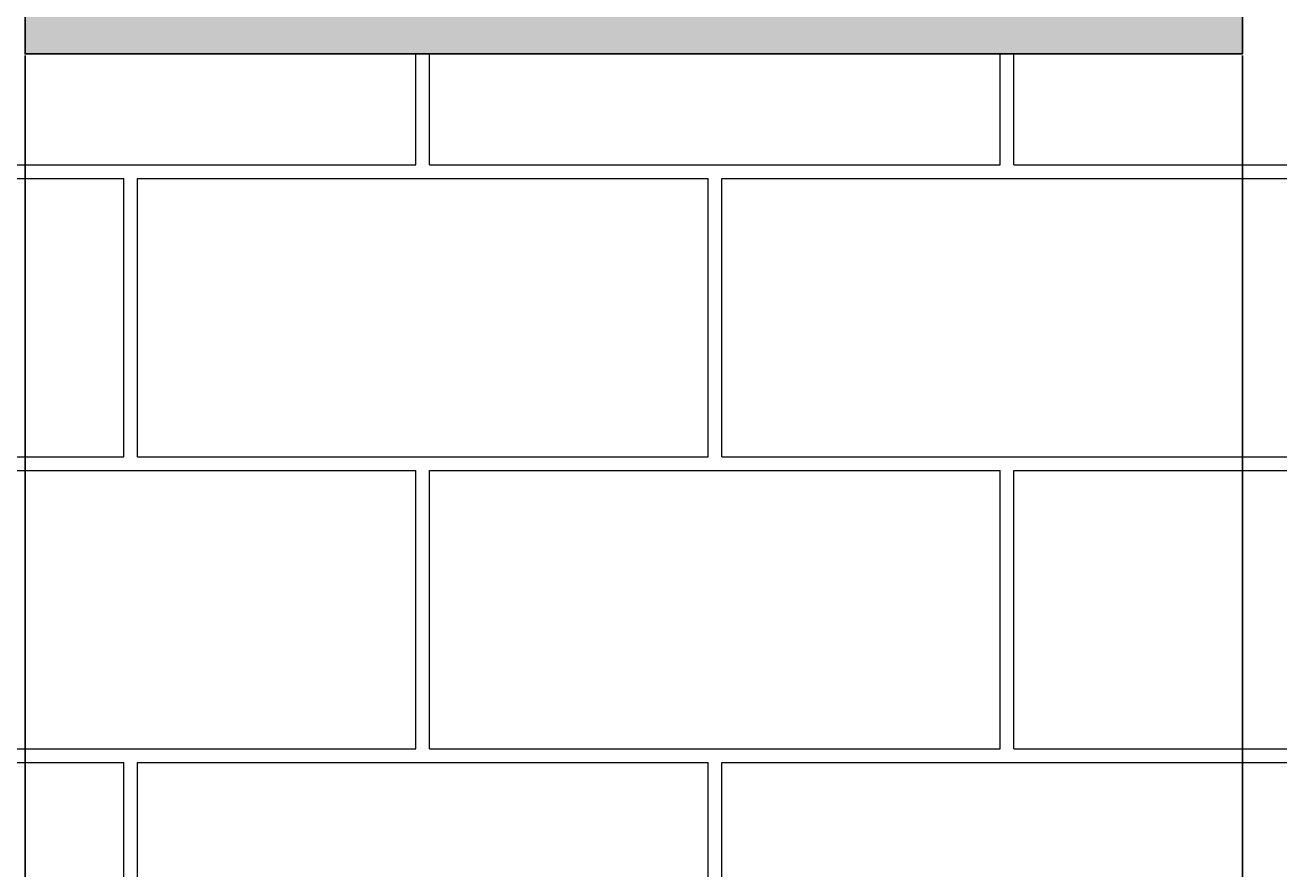
# Model space of a CAD drawing. Units: inches. Extents: x -301 to 715, y -607 to 364.
# Tile 132 of 141: x 310 to 362, y -475 to -440. Entities that reach past the tile are written whole.
import ezdxf

# ---------------------------------------------------------------- set-up
doc = ezdxf.new("R2010")
doc.units = ezdxf.units.IN
doc.header["$MEASUREMENT"] = 0
for name, color, linetype, lineweight in [('A-ANNO-DIMS', 2, 'Continuous', 18), ('A-ELEV-PATT', 4, 'Continuous', 13), ('A-GLAZ', 2, 'Continuous', 25)]:
    doc.layers.add(name, color=color, linetype=linetype, lineweight=lineweight)
doc.styles.get("Standard").update_dxf_attribs({"font": 'arial.ttf'})
doc.dimstyles.get("Standard").update_dxf_attribs({"dimtxt": 0.18, "dimasz": 0.18, "dimexe": 0.18, "dimexo": 0.0625, "dimgap": 0.09, "dimtad": 0, "dimtih": 1, "dimtoh": 1, "dimdec": 1, "dimzin": 0, "dimdsep": 46, "dimlunit": 4, "dimtxsty": 'Standard', "dimcen": 0.09, "dimclrd": 3, "dimclre": 4, "dimclrt": 6, "dimadec": 0, "dimazin": 0, "dimtfac": 1, "dimtdec": 1, "dimtofl": 0, "dimtmove": 0, "dimatfit": 3, "dimfxl": 1, "dimtfill": 2, "dimtfillclr": 51, "dimtolj": 1, "dimtzin": 0, "dimarcsym": 0})

# ---------------------------------------------------------------- blocks, each defined once
blk = doc.blocks.new('*D195')
at = {"layer": 'A-ANNO-DIMS', "color": 4, "lineweight": -2, "transparency": 16777216}
for p, q in [((310.018, -441.615), (310.018, -606.789)), ((360.018, -441.615), (360.018, -606.789))]:
    blk.add_line(p, q, dxfattribs=at)
at = {"layer": 'A-ANNO-DIMS', "color": 3, "lineweight": -2, "transparency": 16777216}
for p, q in [((310.198, -606.609), (334.685, -606.609)), ((359.838, -606.609), (335.351, -606.609))]:
    blk.add_line(p, q, dxfattribs=at)
at = {"layer": 'A-ANNO-DIMS', "color": 3, "transparency": 16777216}
for points in [[(310.198, -606.579), (310.198, -606.639), (310.018, -606.609)], [(359.838, -606.579), (359.838, -606.639), (360.018, -606.609)]]:
    blk.add_solid(points, dxfattribs=at)
at = {"layer": 'Defpoints', "color": 0, "transparency": 16777216}
for p in [(310.018, -441.552), (360.018, -441.552), (360.018, -606.609)]:
    blk.add_point(p, dxfattribs=at)
at = {"layer": 'A-ANNO-DIMS', "color": 6, "transparency": 16777216, "insert": (335.018, -606.609), "char_height": 0.18, "attachment_point": 5, "bg_fill": 1, "box_fill_scale": 1.25, "bg_fill_color": 51, "bg_fill_transparency": 0}
blk.add_mtext('\\A1;4\'-2"', dxfattribs=at)
blk = doc.blocks.new('*D196')
at = {"layer": 'A-ANNO-DIMS', "color": 4, "lineweight": -2, "transparency": 16777216}
for p, q in [((360.018, -441.615), (360.018, -606.789)), ((413.018, -489.615), (413.018, -606.789))]:
    blk.add_line(p, q, dxfattribs=at)
at = {"layer": 'A-ANNO-DIMS', "color": 3, "lineweight": -2, "transparency": 16777216}
for p, q in [((360.198, -606.609), (386.185, -606.609)), ((412.838, -606.609), (386.851, -606.609))]:
    blk.add_line(p, q, dxfattribs=at)
at = {"layer": 'A-ANNO-DIMS', "color": 3, "transparency": 16777216}
for points in [[(360.198, -606.579), (360.198, -606.639), (360.018, -606.609)], [(412.838, -606.579), (412.838, -606.639), (413.018, -606.609)]]:
    blk.add_solid(points, dxfattribs=at)
at = {"layer": 'Defpoints', "color": 0, "transparency": 16777216}
for p in [(360.018, -441.552), (413.018, -489.552), (413.018, -606.609)]:
    blk.add_point(p, dxfattribs=at)
at = {"layer": 'A-ANNO-DIMS', "color": 6, "transparency": 16777216, "insert": (386.518, -606.609), "char_height": 0.18, "attachment_point": 5, "bg_fill": 1, "box_fill_scale": 1.25, "bg_fill_color": 51, "bg_fill_transparency": 0}
blk.add_mtext('\\A1;4\'-5"', dxfattribs=at)
blk = doc.blocks.new('*D200')
at = {"layer": 'A-ANNO-DIMS', "color": 4, "lineweight": -2, "transparency": 16777216}
for p, q in [((412.955, -393.552), (121.926, -393.552)), ((412.955, -489.552), (121.926, -489.552))]:
    blk.add_line(p, q, dxfattribs=at)
at = {"layer": 'A-ANNO-DIMS', "color": 3, "lineweight": -2, "transparency": 16777216}
for p, q in [((122.106, -393.732), (122.106, -441.371)), ((122.106, -489.372), (122.106, -441.734))]:
    blk.add_line(p, q, dxfattribs=at)
at = {"layer": 'A-ANNO-DIMS', "color": 3, "transparency": 16777216}
for points in [[(122.076, -393.732), (122.136, -393.732), (122.106, -393.552)], [(122.076, -489.372), (122.136, -489.372), (122.106, -489.552)]]:
    blk.add_solid(points, dxfattribs=at)
at = {"layer": 'Defpoints', "color": 0, "transparency": 16777216}
for p in [(122.106, -393.552), (413.018, -393.552), (413.018, -489.552)]:
    blk.add_point(p, dxfattribs=at)
at = {"layer": 'A-ANNO-DIMS', "color": 6, "transparency": 16777216, "insert": (122.106, -441.552), "char_height": 0.18, "attachment_point": 5, "bg_fill": 1, "box_fill_scale": 1.25, "bg_fill_color": 51, "bg_fill_transparency": 0}
blk.add_mtext('\\A1;8\'-0"', dxfattribs=at)

msp = doc.modelspace()

# ---------------------------------------------------------------- hatches: boundary and pattern name
at = {"layer": 'A-ELEV-PATT'}
h = msp.add_hatch(color=256, dxfattribs=at)
h.dxf.hatch_style = 1
h.paths.add_polyline_path([(591.518, -363.552), (254.018, -363.552), (254.018, -369.552), (591.518, -369.552)])
h.paths.add_polyline_path([(461.018, -393.552), (413.018, -393.552), (413.018, -489.552), (461.018, -489.552)])
h.paths.add_polyline_path([(456.018, -398.552), (456.018, -484.552), (418.018, -484.552), (418.018, -398.552)], flags=16)
h.paths.add_polyline_path([(546.768, -393.552), (496.768, -393.552), (496.768, -441.552), (546.768, -441.552)])
h.paths.add_polyline_path([(501.768, -398.552), (541.768, -398.552), (541.768, -436.552), (501.768, -436.552)], flags=16)
h.paths.add_polyline_path([(360.018, -393.552), (310.018, -393.552), (310.018, -441.552), (360.018, -441.552)])
h.paths.add_polyline_path([(355.018, -398.552), (355.018, -436.552), (315.018, -436.552), (315.018, -398.552)], flags=16)
h = msp.add_hatch(dxfattribs=at)
h.set_pattern_fill('AR-B816C', color=256, scale=1.5)
h.set_pattern_definition([(0, (458.621, 9.325), (12, 12), [23.4375, -0.5625]), (0, (446.621, 9.887), (12, 12), [23.4375, -0.5625]), (90, (458.621, 9.325), (-12, 12), [-12.5625, 11.4375]), (90, (458.059, 9.325), (-12, 12), [-12.5625, 11.4375])])
h.paths.add_polyline_path([(254.018, -489.552), (413.018, -489.552), (413.018, -393.552), (461.018, -393.552), (461.018, -489.552), (591.518, -489.552), (591.518, -369.552), (254.018, -369.552)])
h.paths.add_polyline_path([(310.018, -393.552), (360.018, -393.552), (360.018, -441.552), (310.018, -441.552)], flags=16)
h.paths.add_polyline_path([(315.018, -398.552), (355.018, -398.552), (355.018, -436.552), (315.018, -436.552)], flags=0)
h.paths.add_polyline_path([(496.768, -393.552), (546.768, -393.552), (546.768, -441.552), (496.768, -441.552)], flags=16)
h.paths.add_polyline_path([(501.768, -398.552), (541.768, -398.552), (541.768, -436.552), (501.768, -436.552)], flags=0)

# ---------------------------------------------------------------- linework, layer by layer
at = {"layer": 'A-GLAZ'}
msp.add_lwpolyline([(310.018, -393.552), (360.018, -393.552), (360.018, -441.552), (310.018, -441.552)], close=True, dxfattribs=at)

# ---------------------------------------------------------------- dimensions: what is measured, and where the dimension line sits
at = {"layer": 'A-ANNO-DIMS'}
dim = msp.add_linear_dim(base=(122.106, -393.552), p1=(413.018, -489.552), p2=(413.018, -393.552), angle=90, dimstyle='Standard', override={"dimdec": 1, "dimlfac": 1, "dimrnd": 0, "dimzin": 1, "dimdsep": 46, "dimlunit": 4, "dimfrac": 2}, dxfattribs=at)
dim.commit()
dim.dimension.update_dxf_attribs({"geometry": '*D200', "text_midpoint": (122.106, -441.552)})
for base, p1, p2, picture, middle in [((360.018, -606.609), (310.018, -441.552), (360.018, -441.552), '*D195', (335.018, -606.609)), ((413.018, -606.609), (360.018, -441.552), (413.018, -489.552), '*D196', (386.518, -606.609))]:
    dim = msp.add_linear_dim(base=base, p1=p1, p2=p2, dimstyle='Standard', override={"dimdec": 1, "dimlfac": 1, "dimrnd": 0, "dimzin": 1, "dimdsep": 46, "dimlunit": 4, "dimfrac": 2}, dxfattribs=at)
    dim.commit()
    dim.dimension.update_dxf_attribs({"geometry": picture, "text_midpoint": middle})

doc.saveas('drawing.dxf')
